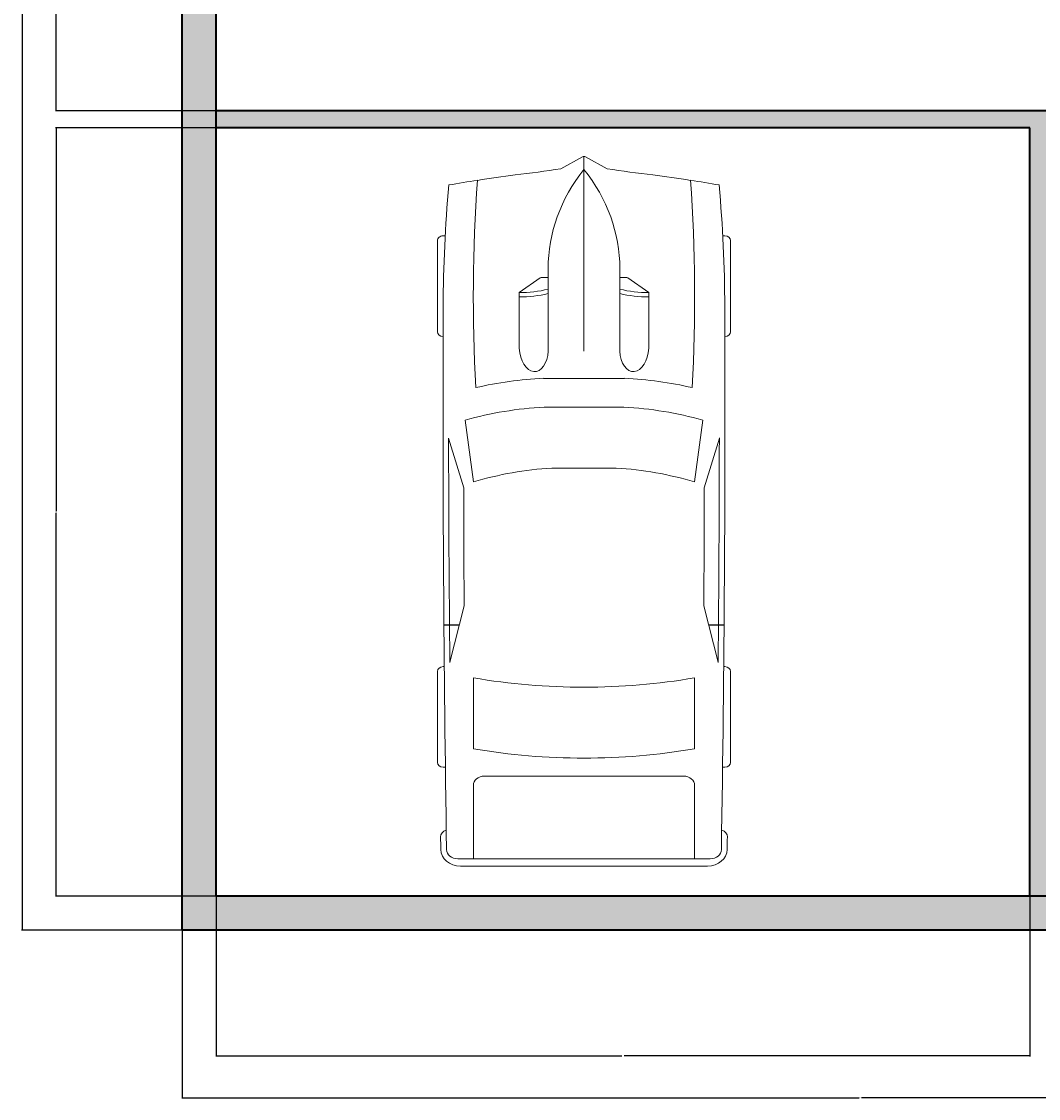
# Model space of a CAD drawing. Units: inches. Extents: x 1563 to 2428, y 777 to 1464.
# Tile 1 of 11: x 1563 to 1832, y 777 to 1063. Entities that reach past the tile are written whole.
import ezdxf

# ---------------------------------------------------------------- set-up
doc = ezdxf.new("R2010")
doc.units = ezdxf.units.IN
for name, color, linetype, lineweight in [('A-ANNO-DIMS', 2, 'Continuous', 18), ('A-FLOR-EDGE', 7, 'Continuous', 25), ('A-SITE-VEHI', 8, 'Continuous', 13), ('A-WALL', 7, 'Continuous', 35), ('A-WALL-PATT', 8, 'Continuous', 13)]:
    doc.layers.add(name, color=color, linetype=linetype, lineweight=lineweight)
doc.styles.get("Standard").update_dxf_attribs({"font": 'arial.ttf'})
doc.dimstyles.get("Standard").update_dxf_attribs({"dimtxt": 0.18, "dimasz": 0.18, "dimexe": 0.18, "dimexo": 0.0625, "dimgap": 0.09, "dimtad": 0, "dimtih": 1, "dimtoh": 1, "dimdec": 4, "dimzin": 0, "dimdsep": 46, "dimtxsty": 'Standard', "dimcen": 0.09, "dimadec": 0, "dimazin": 0, "dimtfac": 1, "dimtdec": 4, "dimtofl": 0, "dimtmove": 0, "dimatfit": 3, "dimfxl": 1, "dimtolj": 1, "dimtzin": 0, "dimarcsym": 0})

# ---------------------------------------------------------------- blocks, each defined once
blk = doc.blocks.new('*U6')
for p, q in [((21.1, 37.41), (21.1, 36.83)), ((46.55, 38.89), (22.35, 38.89)), ((47.8, 37.39), (47.8, 37.41)), ((135.45, 37.07), (135.45, 37.41)), ((136.7, 38.89), (160.9, 38.89)), ((162.15, 37.41), (162.15, 36.77)), ((87.99, 31.87), (74.76, 35.92)), ((134.31, 35.6), (119.29, 31.78)), ((70.03, 31.54), (86.41, 29.35)), ((186.47, -33.5), (186.47, 33.5)), ((188.4, -32.76), (188.4, 32.76)), ((138.42, 29.35), (157.25, 29.35)), ((186.47, 29.35), (167.01, 29.35)), ((164.52, 26.39), (164.52, -26.39)), ((32.27, 11.63), (36.13, 17.17)), ((36.13, 17.17), (50.94, 17.17)), ((29.77, 9.51), (51.68, 9.51)), ((32.12, 9.51), (32.12, 11.15)), ((58.92, -10.77), (58.92, 10.77)), ((66.55, -10.53), (66.55, 10.53)), ((186.47, -10.53), (186.47, 10.53)), ((3.27, 6.13), (0.1, 0.41)), ((82.74, 8.5), (82.74, -8.5)), ((0, 0), (51.68, 0)), ((0.1, -0.41), (3.27, -6.13)), ((29.77, -9.51), (51.68, -9.51)), ((32.12, -9.51), (32.12, -11.15)), ((32.27, -11.63), (36.13, -17.17)), ((36.13, -17.17), (50.94, -17.17)), ((86.41, -29.35), (70.03, -31.54)), ((157.25, -29.35), (138.42, -29.35)), ((167.01, -29.35), (186.47, -29.35)), ((87.99, -31.87), (74.76, -35.92)), ((134.31, -35.6), (119.29, -31.78)), ((21.1, -37.41), (21.1, -36.83)), ((135.45, -37.07), (135.45, -37.41)), ((162.15, -37.41), (162.15, -36.77)), ((46.55, -38.89), (22.35, -38.89)), ((47.8, -37.39), (47.8, -37.41)), ((136.7, -38.89), (160.9, -38.89))]:
    blk.add_line(p, q)
for centre, major_axis, ratio, start_param, end_param in [((41.19, -490.86), (0, 528.23), 0.842304, 0.00281, 0.075598), ((22.35, 37.41), (0, -1.48), 0.842304, 3.141593, 4.712389), ((64.48, -10555.62), (0, 10593.03), 0.842304, -0.013397, 0.002797), ((46.55, 37.41), (0, 1.48), 0.842304, -1.570796, 0), ((136.7, 37.41), (0, -1.48), 0.842304, 3.141593, 4.712389), ((160.9, 37.41), (0, 1.48), 0.842304, -1.570796, 0), ((180.63, 35.84), (0, 2.22), 0.842304, -0.013017, 1.249894), ((64.48, -10556.36), (0, 10595.31), 0.842304, -0.013397, -0.013017), ((183.98, 32.76), (0, -5.25), 0.842304, 1.570796, 3.128196), ((266.03, -27.52), (0, 313.31), 0.842304, 1.367076, 1.39176), ((64.48, -10555.62), (0, -10591.55), 0.842304, 3.133765, 3.140441), ((183.98, 33.5), (0, -2.96), 0.842304, 1.570796, 3.128196), ((135.29, 5.39), (0, 81.77), 0.842304, 1.245306, 1.50788), ((95.79, -3666.35), (0, -3698.24), 0.842304, 3.134049, 3.144098), ((37.47, -593.96), (0, -623.33), 0.842304, 3.096046, 3.200911), ((134.4, 5.39), (0, -89.78), 0.842304, 4.449482, 4.652344), ((149.6, 2.8), (0, -79.58), 0.842304, 4.372215, 4.640744), ((17.08, 0), (0, 147.02), 0.842304, 4.511394, 4.913384), ((35.91, 0), (0, 147.02), 0.842304, 4.511394, 4.913384), ((167.01, 26.39), (0, 2.96), 0.842304, 0, 1.570796), ((259.18, -27.52), (0, -305.3), 0.842304, 4.528606, 4.561838), ((-204.49, 52.4), (0, -250.96), 0.842304, 1.385369, 1.434372), ((13.04, 17.01), (0, 27.42), 0.842304, 4.435146, 4.718221), ((14.2, 17.01), (0, 27.42), 0.842304, 4.435146, 4.718221), ((50.79, 13.34), (6.34, -0.36), 0.603834, -1.395552, 1.581315), ((32.75, 11.15), (0, 0.74), 0.842304, 0.879714, 1.570796), ((29.77, -46.66), (0, 56.17), 0.842304, 0, 0.590319), ((0.62, 0), (0, -0.74), 0.842304, 4.131459, 5.293319), ((29.77, 46.66), (0, 56.17), 0.842304, 2.551274, 3.141593), ((-204.49, -52.4), (0, 250.96), 0.842304, -1.434372, -1.385369), ((149.6, -2.8), (0, -79.58), 0.842304, -1.499151, -1.230623), ((32.75, -11.15), (0, -0.74), 0.842304, 4.712389, 5.403472), ((13.04, -17.01), (0, -27.42), 0.842304, 1.564964, 1.848039), ((14.2, -17.01), (0, -27.42), 0.842304, 1.564964, 1.848039), ((134.4, -5.39), (0, -89.78), 0.842304, -1.510751, -1.307889), ((135.29, -5.39), (0, -81.77), 0.842304, -1.50788, -1.245306), ((259.18, 27.52), (0, 305.3), 0.842304, 1.721348, 1.754579), ((266.03, 27.52), (0, 313.31), 0.842304, 1.749832, 1.774517), ((37.47, 593.96), (0, -623.33), 0.842304, -0.059319, 0.045547), ((167.01, -26.39), (0, -2.96), 0.842304, 4.712389, 6.283185), ((95.79, 3666.35), (0, -3698.24), 0.842304, -0.002505, 0.007544), ((183.98, -33.5), (0, 2.96), 0.842304, 3.15499, 4.712389), ((183.98, -32.76), (0, -5.25), 0.842304, 0.013397, 1.570796), ((41.19, 490.86), (0, -528.23), 0.842304, -0.075598, -0.00281), ((64.48, 10555.62), (0, 10593.03), 0.842304, 3.138796, 3.15499), ((64.48, 10555.62), (0, -10591.55), 0.842304, 0.001152, 0.007828), ((180.63, -35.84), (0, -2.22), 0.842304, -1.249894, 0.013017), ((22.35, -37.41), (0, 1.48), 0.842304, 1.570796, 3.141593), ((46.55, -37.41), (0, -1.48), 0.842304, 0, 1.570796), ((136.7, -37.41), (0, -1.48), 0.842304, -1.570796, 0), ((160.9, -37.41), (0, 1.48), 0.842304, 3.141593, 4.712389), ((64.48, 10556.36), (0, 10595.31), 0.842304, 3.15461, 3.15499)]:
    blk.add_ellipse(centre, major_axis=major_axis, ratio=ratio, start_param=start_param, end_param=end_param)
at = {"extrusion": (0, 0, -1)}
blk.add_ellipse((50.79, -13.34), major_axis=(6.34, 0.36), ratio=0.603834, start_param=-1.395552, end_param=1.581315, dxfattribs=at)
blk = doc.blocks.new('*D48')
at = {"layer": 'A-ANNO-DIMS', "color": 0, "lineweight": -2, "transparency": 16777216}
for p, q in [((1605.11, 821.37), (1605.11, 776.74)), ((1965.11, 821.37), (1965.11, 776.74)), ((1605.29, 776.92), (1784.82, 776.92)), ((1964.93, 776.92), (1785.39, 776.92))]:
    blk.add_line(p, q, dxfattribs=at)
at = {"layer": 'A-ANNO-DIMS', "color": 0, "transparency": 16777216}
for points in [[(1605.29, 776.95), (1605.29, 776.89), (1605.11, 776.92)], [(1964.93, 776.95), (1964.93, 776.89), (1965.11, 776.92)]]:
    blk.add_solid(points, dxfattribs=at)
at = {"layer": 'Defpoints', "color": 0, "transparency": 16777216}
for p in [(1605.11, 821.43), (1965.11, 821.43), (1965.11, 776.92)]:
    blk.add_point(p, dxfattribs=at)
at = {"layer": 'A-ANNO-DIMS', "color": 0, "transparency": 16777216, "insert": (1785.11, 776.92), "char_height": 0.18, "attachment_point": 5}
blk.add_mtext('\\A1;360', dxfattribs=at)
blk = doc.blocks.new('*D49')
at = {"layer": 'A-ANNO-DIMS', "color": 0, "lineweight": -2, "transparency": 16777216}
for p, q in [((1605.04, 1421.43), (1562.53, 1421.43)), ((1562.71, 1421.25), (1562.71, 1121.61)), ((1562.71, 821.61), (1562.71, 1121.25)), ((1605.04, 821.43), (1562.53, 821.43))]:
    blk.add_line(p, q, dxfattribs=at)
at = {"layer": 'A-ANNO-DIMS', "color": 0, "transparency": 16777216}
for points in [[(1562.68, 1421.25), (1562.74, 1421.25), (1562.71, 1421.43)], [(1562.68, 821.61), (1562.74, 821.61), (1562.71, 821.43)]]:
    blk.add_solid(points, dxfattribs=at)
at = {"layer": 'Defpoints', "color": 0, "transparency": 16777216}
for p in [(1562.71, 1421.43), (1605.11, 1421.43), (1605.11, 821.43)]:
    blk.add_point(p, dxfattribs=at)
at = {"layer": 'A-ANNO-DIMS', "color": 0, "transparency": 16777216, "insert": (1562.71, 1121.43), "char_height": 0.18, "attachment_point": 5}
blk.add_mtext('\\A1;600', dxfattribs=at)
blk = doc.blocks.new('*D58')
at = {"layer": 'A-ANNO-DIMS', "color": 0, "lineweight": -2, "transparency": 16777216}
for p, q in [((1614.04, 1199.43), (1571.53, 1199.43)), ((1571.71, 1199.25), (1571.71, 1119.36)), ((1571.71, 1039.11), (1571.71, 1119)), ((1614.04, 1038.93), (1571.53, 1038.93))]:
    blk.add_line(p, q, dxfattribs=at)
at = {"layer": 'A-ANNO-DIMS', "color": 0, "transparency": 16777216}
for points in [[(1571.68, 1199.25), (1571.74, 1199.25), (1571.71, 1199.43)], [(1571.68, 1039.11), (1571.74, 1039.11), (1571.71, 1038.93)]]:
    blk.add_solid(points, dxfattribs=at)
at = {"layer": 'Defpoints', "color": 0, "transparency": 16777216}
for p in [(1571.71, 1199.43), (1614.11, 1199.43), (1614.11, 1038.93)]:
    blk.add_point(p, dxfattribs=at)
at = {"layer": 'A-ANNO-DIMS', "color": 0, "transparency": 16777216, "insert": (1571.71, 1119.18), "char_height": 0.18, "attachment_point": 5}
blk.add_mtext('\\A1;160.5', dxfattribs=at)
blk = doc.blocks.new('*D59')
at = {"layer": 'A-ANNO-DIMS', "color": 0, "lineweight": -2, "transparency": 16777216}
for p, q in [((1614.04, 1034.43), (1571.53, 1034.43)), ((1571.71, 1034.25), (1571.71, 932.61)), ((1571.71, 830.61), (1571.71, 932.25)), ((1614.04, 830.43), (1571.53, 830.43))]:
    blk.add_line(p, q, dxfattribs=at)
at = {"layer": 'A-ANNO-DIMS', "color": 0, "transparency": 16777216}
for points in [[(1571.68, 1034.25), (1571.74, 1034.25), (1571.71, 1034.43)], [(1571.68, 830.61), (1571.74, 830.61), (1571.71, 830.43)]]:
    blk.add_solid(points, dxfattribs=at)
at = {"layer": 'Defpoints', "color": 0, "transparency": 16777216}
for p in [(1571.71, 1034.43), (1614.11, 1034.43), (1614.11, 830.43)]:
    blk.add_point(p, dxfattribs=at)
at = {"layer": 'A-ANNO-DIMS', "color": 0, "transparency": 16777216, "insert": (1571.71, 932.43), "char_height": 0.18, "attachment_point": 5}
blk.add_mtext('\\A1;204', dxfattribs=at)
blk = doc.blocks.new('*D60')
at = {"layer": 'A-ANNO-DIMS', "color": 0, "lineweight": -2, "transparency": 16777216}
for p, q in [((1614.11, 830.37), (1614.11, 787.85)), ((1830.11, 830.37), (1830.11, 787.85)), ((1614.29, 788.03), (1721.82, 788.03)), ((1829.93, 788.03), (1722.4, 788.03))]:
    blk.add_line(p, q, dxfattribs=at)
at = {"layer": 'A-ANNO-DIMS', "color": 0, "transparency": 16777216}
for points in [[(1614.29, 788.06), (1614.29, 788), (1614.11, 788.03)], [(1829.93, 788.06), (1829.93, 788), (1830.11, 788.03)]]:
    blk.add_solid(points, dxfattribs=at)
at = {"layer": 'Defpoints', "color": 0, "transparency": 16777216}
for p in [(1614.11, 830.43), (1830.11, 830.43), (1614.11, 788.03)]:
    blk.add_point(p, dxfattribs=at)
at = {"layer": 'A-ANNO-DIMS', "color": 0, "transparency": 16777216, "insert": (1722.11, 788.03), "char_height": 0.18, "attachment_point": 5}
blk.add_mtext('\\A1;216', dxfattribs=at)

msp = doc.modelspace()

# ---------------------------------------------------------------- hatches: boundary and pattern name
at = {"layer": 'A-WALL-PATT'}
h = msp.add_hatch(color=256, dxfattribs=at)
h.dxf.hatch_style = 1
h.paths.add_polyline_path([(1965.105, 1421.428), (1605.105, 1421.428), (1605.105, 821.428), (1965.105, 821.428)])
h.paths.add_polyline_path([(1614.105, 1199.428), (1704.105, 1199.428), (1738.605, 1199.428), (1738.605, 1251.928), (1734.105, 1251.928), (1734.105, 1203.928), (1704.105, 1203.928), (1614.105, 1203.928), (1614.105, 1335.928), (1665.105, 1335.928), (1665.105, 1340.428), (1614.105, 1340.428), (1614.105, 1412.428), (1704.105, 1412.428), (1704.105, 1340.428), (1701.105, 1340.428), (1701.105, 1335.928), (1704.105, 1335.928), (1768.605, 1335.928), (1768.605, 1340.428), (1708.605, 1340.428), (1708.605, 1412.428), (1807.605, 1412.428), (1807.605, 1340.428), (1804.605, 1340.428), (1804.605, 1335.928), (1807.605, 1335.928), (1807.605, 1275.928), (1815.105, 1275.928), (1815.105, 1280.428), (1812.105, 1280.428), (1812.105, 1412.428), (1956.105, 1412.428), (1956.105, 1280.428), (1854.105, 1280.428), (1854.105, 1275.928), (1956.105, 1275.928), (1956.105, 830.428), (1614.105, 830.428)], flags=16)
h.paths.add_polyline_path([(1917.224, 1038.928), (1917.224, 1043.846, -0.4014527), (1951.591, 1079.751), (1951.591, 1079.786), (1953.163, 1079.786), (1953.163, 1043.846), (1953.163, 1038.455), (1953.105, 1034.428), (1953.105, 1038.928), (1953.163, 1043.846), (1951.591, 1043.846), (1951.591, 1079.751, 0.4014527), (1917.224, 1043.846), (1917.224, 1038.455), (1917.224, 1034.428), (1834.605, 1034.428), (1834.605, 906.928), (1858.605, 906.928), (1858.605, 954.928), (1932.105, 954.928), (1932.105, 902.428), (1834.605, 902.428), (1834.605, 1034.428), (1914.224, 1034.428), (1914.224, 1038.928)], flags=0)
edge = h.paths.add_edge_path(flags=0)
edge.add_ellipse((1674.345, 1004.483), major_axis=(1.48, 0), ratio=0.8423039, start_angle=90, end_angle=180, ccw=False)
edge.add_line((1674.345, 1005.73), (1674.921, 1005.73))
edge.add_ellipse((2202.617, 985.642), major_axis=(528.234, 0), ratio=0.8423039, start_angle=176.34957, end_angle=177.82005, ccw=False)
edge.add_ellipse((1739.278, 760.804), major_axis=(-313.308, 0), ratio=0.8423039, start_angle=-77.87403, end_angle=-76.21947, ccw=False)
edge.add_ellipse((1739.278, 767.659), major_axis=(305.303, 0), ratio=0.8423039, start_angle=100.20954, end_angle=102.44463, ccw=False)
edge.add_ellipse((1659.357, 1231.328), major_axis=(250.96, 0), ratio=0.8423039, start_angle=-80.74343, end_angle=-77.44507)
edge.add_line((1705.625, 1023.567), (1711.685, 1026.918))
edge.add_ellipse((1711.754, 1026.21), major_axis=(0.74, 0), ratio=0.8423039, start_angle=52.06687, end_angle=90, ccw=False)
edge.add_line((1712.16, 1026.731), (1717.882, 1023.567))
edge.add_ellipse((1764.151, 1231.328), major_axis=(250.96, 0), ratio=0.8423039, start_angle=257.44507, end_angle=260.74343)
edge.add_ellipse((1684.229, 767.659), major_axis=(305.303, 0), ratio=0.8423039, start_angle=77.55537, end_angle=79.79046, ccw=False)
edge.add_ellipse((1684.229, 760.804), major_axis=(-313.308, 0), ratio=0.8423039, start_angle=256.21947, end_angle=257.87403, ccw=False)
edge.add_ellipse((1220.891, 985.642), major_axis=(-528.234, 0), ratio=0.8423039, start_angle=182.17995, end_angle=183.65043, ccw=False)
edge.add_line((1748.586, 1005.73), (1749.162, 1005.73))
edge.add_ellipse((1749.162, 1004.483), major_axis=(-1.48, 0), ratio=0.8423039, start_angle=180, end_angle=270, ccw=False)
edge.add_line((1750.642, 1004.483), (1750.642, 980.28))
edge.add_ellipse((1749.162, 980.28), major_axis=(1.48, 0), ratio=0.8423039, start_angle=270, end_angle=360, ccw=False)
edge.add_ellipse((-8843.864, 962.352), major_axis=(10593.026, 0), ratio=0.84230387, start_angle=-0.3241203, end_angle=0.0902291, ccw=False)
edge.add_ellipse((-8843.864, 962.352), major_axis=(10593.026, 0), ratio=0.84230387, start_angle=-0.3838668, end_angle=-0.3241203, ccw=False)
edge.add_ellipse((1749.162, 890.136), major_axis=(1.48, 0), ratio=0.8423039, start_angle=0, end_angle=90, ccw=False)
edge.add_line((1750.642, 890.136), (1750.642, 865.933))
edge.add_ellipse((1749.162, 865.933), major_axis=(1.48, 0), ratio=0.8423039, start_angle=270, end_angle=360, ccw=False)
edge.add_line((1749.162, 864.686), (1748.528, 864.686))
edge.add_ellipse((-8843.864, 962.352), major_axis=(10593.026, 0), ratio=0.84230387, start_angle=-0.6186432, end_angle=-0.5282715, ccw=False)
edge.add_ellipse((1747.592, 846.206), major_axis=(-2.22, 0), ratio=0.8423039, start_angle=179.37176, end_angle=248.46476, ccw=False)
edge.add_ellipse((-8844.604, 962.352), major_axis=(-10595.313, 0), ratio=0.842303864, start_angle=179.3534459, end_angle=179.3717628, ccw=False)
edge.add_ellipse((1744.512, 842.854), major_axis=(-5.246, 0), ratio=0.8423039, start_angle=90, end_angle=179.35345, ccw=False)
edge.add_line((1744.512, 838.435), (1678.995, 838.435))
edge.add_ellipse((1678.995, 842.854), major_axis=(5.246, 0), ratio=0.8423039, start_angle=180.64655, end_angle=270, ccw=False)
edge.add_ellipse((12268.111, 962.352), major_axis=(-10595.313, 0), ratio=0.84230387, start_angle=0.6282372, end_angle=0.6465541, ccw=False)
edge.add_ellipse((1675.916, 846.206), major_axis=(-2.22, 0), ratio=0.8423039, start_angle=-68.46476, end_angle=0.62824, ccw=False)
edge.add_ellipse((12267.371, 962.352), major_axis=(-10593.026, 0), ratio=0.84230387, start_angle=0.5282715, end_angle=0.6465541, ccw=False)
edge.add_line((1674.98, 864.686), (1674.345, 864.686))
edge.add_ellipse((1674.345, 865.933), major_axis=(-1.48, 0), ratio=0.8423039, start_angle=0, end_angle=90, ccw=False)
edge.add_line((1672.865, 865.933), (1672.865, 890.136))
edge.add_ellipse((1674.345, 890.136), major_axis=(1.48, 0), ratio=0.8423039, start_angle=90, end_angle=180, ccw=False)
edge.add_ellipse((12267.371, 962.352), major_axis=(-10593.026, 0), ratio=0.84230387, start_angle=0.3241203, end_angle=0.3838668, ccw=False)
edge.add_ellipse((12267.371, 962.352), major_axis=(-10593.026, 0), ratio=0.84230387, start_angle=-0.0902291, end_angle=0.3241203, ccw=False)
edge.add_ellipse((1674.345, 980.28), major_axis=(-1.48, 0), ratio=0.8423039, start_angle=0, end_angle=90, ccw=False)
edge.add_line((1672.865, 980.28), (1672.865, 1004.483))
h.paths.add_polyline_path([(1622.542, 1135.584), (1648.534, 1136.233), (1648.683, 1130.234), (1647.126, 1130.196), (1648.323, 1082.21), (1649.88, 1082.249), (1650.03, 1076.251), (1624.038, 1075.603, -0.266667)], flags=0)
edge = h.paths.add_edge_path(flags=0)
edge.add_line((1694.584, 990.705), (1700.334, 994.711))
edge.add_line((1700.334, 994.711), (1702.248, 994.711))
edge.add_line((1702.248, 994.711), (1702.248, 997.061))
edge.add_ellipse((1758.417, 997.061), major_axis=(56.169, 0), ratio=0.8423039, start_angle=150.56143, end_angle=180, ccw=False)
edge.add_ellipse((1665.091, 997.061), major_axis=(-56.169, 0), ratio=0.8423039, start_angle=180, end_angle=209.43857, ccw=False)
edge.add_line((1721.26, 997.061), (1721.26, 994.711))
edge.add_line((1721.26, 994.711), (1723.174, 994.711))
edge.add_line((1723.174, 994.711), (1728.923, 990.705))
edge.add_line((1728.923, 990.705), (1728.923, 975.895))
edge.add_ellipse((1725.091, 976.043), major_axis=(0.357, 6.34), ratio=0.6038336, start_angle=106.34259, end_angle=270.99799, ccw=False)
edge.add_line((1721.26, 975.15), (1721.26, 997.061))
edge.add_ellipse((1665.091, 997.061), major_axis=(-56.169, 0), ratio=0.8423039, start_angle=180, end_angle=209.43857)
edge.add_ellipse((1758.417, 997.061), major_axis=(56.169, 0), ratio=0.8423039, start_angle=150.56143, end_angle=180)
edge.add_line((1702.248, 997.061), (1702.248, 975.15))
edge.add_ellipse((1698.416, 976.043), major_axis=(-0.357, 6.34), ratio=0.6038336, start_angle=89.00201, end_angle=253.65741, ccw=False)
edge.add_line((1694.584, 975.895), (1694.584, 990.705))
edge = h.paths.add_edge_path(flags=0)
edge.add_line((1675.832, 952.075), (1679.883, 938.848))
edge.add_ellipse((5378.107, 931.045), major_axis=(-3698.236, 0), ratio=0.84230387, start_angle=-0.120897, end_angle=0.364076)
edge.add_line((1679.976, 907.545), (1676.149, 892.52))
edge.add_ellipse((12267.371, 962.352), major_axis=(10591.546, 0), ratio=0.84230387, start_angle=180.3241656, end_angle=180.3777642, ccw=False)
edge.add_ellipse((12267.371, 962.352), major_axis=(10591.546, 0), ratio=0.84230387, start_angle=180.0555943, end_angle=180.3241656, ccw=False)
edge = h.paths.add_edge_path(flags=0)
edge.add_ellipse((1706.366, 891.542), major_axis=(81.773, 0), ratio=0.8423039, start_angle=94.27742, end_angle=111.83495, ccw=False)
edge.add_line((1701.225, 960.283), (1722.283, 960.283))
edge.add_ellipse((1717.141, 891.542), major_axis=(-81.773, 0), ratio=0.8423039, start_angle=248.16505, end_angle=265.72258, ccw=False)
edge.add_line((1743.29, 956.803), (1741.105, 940.427))
edge.add_ellipse((1714.553, 877.238), major_axis=(79.58, 0), ratio=0.8423039, start_angle=67.20809, end_angle=85.12993)
edge.add_line((1720.25, 944.097), (1703.258, 944.097))
edge.add_ellipse((1708.954, 877.238), major_axis=(79.58, 0), ratio=0.8423039, start_angle=94.87007, end_angle=112.79191)
edge.add_line((1682.403, 940.427), (1680.218, 956.803))
h.paths.add_polyline_path([(1664.992, 1093.991), (1664.992, 1123.991), (1724.992, 1123.991), (1724.992, 1093.991)], flags=0)
h.paths.add_polyline_path([(1716.588, 1099.729), (1715.404, 1099.805), (1715.021, 1099.823), (1716.177, 1099.758)], flags=0)
h.paths.add_polyline_path([(1711.325, 1103.757), (1712.167, 1103.706), (1713.009, 1103.642), (1713.84, 1103.566), (1715.041, 1103.439), (1716.532, 1103.244), (1717.793, 1103.048), (1718.876, 1102.854), (1719.676, 1102.699), (1720.157, 1102.605), (1720.632, 1102.513), (1721.109, 1102.424), (1721.595, 1102.339), (1722.088, 1102.264), (1722.585, 1102.205), (1723.082, 1102.17), (1723.575, 1102.164), (1724.321, 1102.211), (1724.533, 1102.268), (1723.842, 1102.16), (1722.864, 1102.172), (1721.894, 1102.287), (1720.935, 1102.454), (1720.157, 1102.605), (1719.676, 1102.699), (1719.18, 1102.795), (1718.66, 1102.892), (1718.109, 1102.991), (1717.517, 1103.091), (1716.876, 1103.191), (1716.179, 1103.29), (1715.435, 1103.387), (1714.652, 1103.48), (1713.84, 1103.566), (1713.009, 1103.642), (1712.167, 1103.706), (1711.325, 1103.757), (1710.492, 1103.791), (1709.676, 1103.806), (1708.873, 1103.805), (1707.707, 1103.78), (1707.292, 1103.757), (1708.499, 1103.805), (1710.086, 1103.807)], flags=0)
h.paths.add_polyline_path([(1713.959, 1106.591), (1714.651, 1106.624), (1715.279, 1106.674), (1715.852, 1106.736), (1716.373, 1106.807), (1716.851, 1106.885), (1717.289, 1106.966), (1717.696, 1107.046), (1718.341, 1107.178), (1719.173, 1107.331), (1720.169, 1107.421), (1721.131, 1107.383), (1722.032, 1107.286), (1722.934, 1107.152), (1723.887, 1106.983), (1724.746, 1106.795), (1724.72, 1106.798), (1724.663, 1106.807), (1724.241, 1106.906), (1724.159, 1106.924), (1723.885, 1106.979), (1723.546, 1107.044), (1723.157, 1107.113), (1722.732, 1107.182), (1722.284, 1107.249), (1721.827, 1107.308), (1721.375, 1107.357), (1720.942, 1107.391), (1720.539, 1107.406), (1720.162, 1107.405), (1719.804, 1107.388), (1719.459, 1107.357), (1719.12, 1107.314), (1718.781, 1107.259), (1718.435, 1107.195), (1718.076, 1107.124), (1717.402, 1106.986), (1716.59, 1106.837), (1715.56, 1106.696), (1714.317, 1106.598)], flags=0)
h.paths.add_polyline_path([(1708.692, 1110.124), (1709.455, 1110.13), (1710.147, 1110.149), (1710.772, 1110.18), (1711.334, 1110.224), (1711.836, 1110.28), (1712.283, 1110.349), (1712.678, 1110.43), (1713.026, 1110.524), (1713.33, 1110.63), (1713.596, 1110.746), (1713.832, 1110.87), (1714.042, 1110.999), (1714.234, 1111.131), (1714.413, 1111.264), (1714.586, 1111.396), (1715.065, 1111.75), (1715.879, 1112.11), (1716.842, 1112.224), (1717.903, 1112.165), (1719.048, 1111.965), (1719.867, 1111.736), (1720.686, 1111.487), (1721.596, 1111.22), (1721.917, 1111.136), (1721.028, 1111.383), (1720.222, 1111.628), (1719.815, 1111.75), (1719.434, 1111.857), (1719.054, 1111.951), (1718.672, 1112.031), (1718.292, 1112.097), (1717.918, 1112.149), (1717.554, 1112.185), (1717.204, 1112.204), (1716.871, 1112.206), (1716.559, 1112.191), (1716.271, 1112.156), (1716.006, 1112.105), (1715.761, 1112.038), (1715.534, 1111.957), (1715.323, 1111.864), (1715.125, 1111.759), (1714.937, 1111.645), (1714.759, 1111.524), (1714.586, 1111.396), (1714.413, 1111.264), (1714.003, 1110.96), (1713.331, 1110.606), (1712.501, 1110.382), (1711.61, 1110.245), (1710.489, 1110.158), (1709.111, 1110.121)], flags=0)
h.paths.add_polyline_path([(1707.127, 1113.075), (1707.639, 1113.025), (1708.092, 1112.991), (1708.49, 1112.975), (1708.836, 1112.977), (1709.135, 1112.996), (1709.392, 1113.032), (1709.612, 1113.084), (1709.798, 1113.15), (1709.957, 1113.23), (1710.092, 1113.324), (1710.208, 1113.431), (1710.304, 1113.554), (1710.379, 1113.698), (1710.434, 1113.866), (1710.467, 1114.062), (1710.477, 1114.289), (1710.463, 1114.553), (1710.426, 1114.857), (1710.364, 1115.202), (1710.282, 1115.58), (1710.184, 1115.98), (1710.076, 1116.391), (1709.961, 1116.801), (1709.844, 1117.201), (1709.731, 1117.579), (1709.626, 1117.924), (1709.532, 1118.228), (1709.454, 1118.493), (1709.392, 1118.723), (1709.351, 1118.924), (1709.293, 1119.435), (1709.831, 1119.942), (1710.705, 1120.121), (1711.507, 1119.898), (1712.224, 1119.567), (1713.189, 1119.016), (1713.529, 1118.804), (1712.958, 1119.148), (1712.468, 1119.428), (1712.046, 1119.649), (1711.683, 1119.817), (1711.366, 1119.937), (1711.084, 1120.016), (1710.826, 1120.057), (1710.582, 1120.067), (1710.354, 1120.049), (1710.142, 1120.006), (1709.951, 1119.941), (1709.781, 1119.857), (1709.635, 1119.757), (1709.516, 1119.645), (1709.426, 1119.524), (1709.366, 1119.395), (1709.335, 1119.255), (1709.331, 1119.1), (1709.351, 1118.924), (1709.392, 1118.723), (1709.454, 1118.493), (1709.52, 1118.268), (1709.799, 1117.356), (1710.028, 1116.57), (1710.245, 1115.749), (1710.45, 1114.804), (1710.477, 1114.289), (1710.448, 1113.654), (1709.908, 1113.153), (1709.165, 1112.979), (1708.318, 1112.974), (1707.448, 1113.039)], flags=0)
h.paths.add_polyline_path([(1700.892, 1119.857), (1701.604, 1119.819), (1702.196, 1119.805), (1702.683, 1119.813), (1703.076, 1119.841), (1703.387, 1119.887), (1703.63, 1119.951), (1703.816, 1120.03), (1703.959, 1120.124), (1704.069, 1120.23), (1704.15, 1120.346), (1704.204, 1120.47), (1704.234, 1120.599), (1704.242, 1120.731), (1704.231, 1120.864), (1704.202, 1120.996), (1704.159, 1121.124), (1704.103, 1121.246), (1704.039, 1121.362), (1703.97, 1121.474), (1703.901, 1121.582), (1703.834, 1121.687), (1703.775, 1121.79), (1703.564, 1122.226), (1704.048, 1122.698), (1704.756, 1122.769), (1705.49, 1122.723), (1706.24, 1122.641), (1706.547, 1122.601), (1706.092, 1122.657), (1705.695, 1122.701), (1705.348, 1122.732), (1705.049, 1122.751), (1704.792, 1122.757), (1704.573, 1122.751), (1704.386, 1122.732), (1704.227, 1122.701), (1704.092, 1122.657), (1703.977, 1122.601), (1703.88, 1122.534), (1703.802, 1122.458), (1703.742, 1122.374), (1703.702, 1122.284), (1703.68, 1122.188), (1703.677, 1122.09), (1703.692, 1121.991), (1703.726, 1121.89), (1703.769, 1121.802), (1704.039, 1121.362), (1704.301, 1120.887), (1704.133, 1120.165), (1703.43, 1119.866), (1702.481, 1119.798), (1701.306, 1119.827)], flags=0)
edge = h.paths.add_edge_path(flags=0)
edge.add_ellipse((1711.754, 1009.752), major_axis=(-147.018, 0), ratio=0.8423039, start_angle=76.40187, end_angle=103.59813)
edge.add_line((1741.105, 888.411), (1741.105, 869.587))
edge.add_ellipse((1711.754, 990.928), major_axis=(-147.018, 0), ratio=0.8423039, start_angle=76.40187, end_angle=103.59813, ccw=False)
edge.add_line((1682.403, 869.587), (1682.403, 888.411))
edge = h.paths.add_edge_path(flags=0)
edge.add_ellipse((-8843.864, 962.352), major_axis=(-10591.546, 0), ratio=0.84230387, start_angle=179.6758344, end_angle=179.9444057, ccw=False)
edge.add_ellipse((-8843.864, 962.352), major_axis=(-10591.546, 0), ratio=0.84230387, start_angle=179.6222358, end_angle=179.6758344, ccw=False)
edge.add_line((1747.358, 892.52), (1743.531, 907.545))
edge.add_ellipse((-1954.6, 931.045), major_axis=(3698.236, 0), ratio=0.84230387, start_angle=-0.364076, end_angle=0.120897)
edge.add_line((1743.625, 938.848), (1747.676, 952.075))
h.paths.add_polyline_path([(1637.931, 1162.087), (1637.931, 1188.087, -0.1904762), (1721.931, 1188.087), (1721.931, 1162.087), (1715.931, 1162.087), (1715.931, 1163.644), (1643.931, 1163.644), (1643.931, 1162.087)], flags=0)
h.paths.add_polyline_path([(1667.931, 1189.491, -0.0496282), (1691.931, 1189.491), (1691.931, 1182.705), (1667.931, 1182.705)], flags=0)
edge = h.paths.add_edge_path(flags=0)
edge.add_ellipse((1685.362, 859.825), major_axis=(-2.96, 0), ratio=0.8423039, start_angle=-90, end_angle=0, ccw=False)
edge.add_line((1685.362, 862.318), (1738.145, 862.318))
edge.add_ellipse((1738.145, 859.825), major_axis=(2.96, 0), ratio=0.8423039, start_angle=0, end_angle=90, ccw=False)
edge.add_line((1741.105, 859.825), (1741.105, 840.361))
edge.add_line((1741.105, 840.361), (1682.403, 840.361))
edge.add_line((1682.403, 840.361), (1682.403, 859.825))
h.paths.add_polyline_path([(1777.486, 1164.853), (1777.486, 1180.853), (1778.486, 1181.01), (1778.486, 1164.697)], flags=0)
h.paths.add_polyline_path([(1786.986, 1154.853), (1786.986, 1163.369), (1778.986, 1164.619), (1778.986, 1181.088), (1786.986, 1182.338), (1786.986, 1190.853), (1799.502, 1190.853), (1800.752, 1198.853), (1817.221, 1198.853), (1818.471, 1190.853), (1827.502, 1190.853), (1828.752, 1198.853), (1845.221, 1198.853), (1846.471, 1190.853), (1858.986, 1190.853), (1858.986, 1182.338), (1866.986, 1181.088), (1866.986, 1164.619), (1858.986, 1163.369), (1858.986, 1154.853), (1846.471, 1154.853), (1845.221, 1146.853), (1828.752, 1146.853), (1827.502, 1154.853), (1818.471, 1154.853), (1817.221, 1146.853), (1800.752, 1146.853), (1799.502, 1154.853)], flags=0)
h.paths.add_polyline_path([(1800.986, 1145.353), (1800.83, 1146.353), (1817.143, 1146.353), (1816.986, 1145.353)], flags=0)
h.paths.add_polyline_path([(1851.408, 1167.858), (1852.086, 1167.738), (1852.744, 1167.621), (1853.388, 1167.506), (1854.028, 1167.395), (1854.67, 1167.289), (1855.313, 1167.195), (1855.952, 1167.122), (1856.585, 1167.077), (1857.209, 1167.07), (1858.147, 1167.128), (1858.413, 1167.2), (1857.547, 1167.066), (1856.312, 1167.08), (1855.07, 1167.223), (1854.028, 1167.395), (1853.388, 1167.506), (1852.744, 1167.621), (1852.086, 1167.738), (1851.408, 1167.858), (1850.288, 1168.052), (1849.956, 1168.104), (1850.701, 1167.98)], flags=0)
h.paths.add_polyline_path([(1845.435, 1172.646), (1846.222, 1172.707), (1846.941, 1172.785), (1847.601, 1172.874), (1848.21, 1172.971), (1848.777, 1173.072), (1849.311, 1173.173), (1850.14, 1173.331), (1851.063, 1173.483), (1852.014, 1173.591), (1853.012, 1173.633), (1854.075, 1173.594), (1855.251, 1173.473), (1856.4, 1173.306), (1857.391, 1173.132), (1857.945, 1173.02), (1858.196, 1172.965), (1858.595, 1172.871), (1858.575, 1172.874), (1858.49, 1172.894), (1858.371, 1172.924), (1858.196, 1172.965), (1857.945, 1173.02), (1857.602, 1173.089), (1857.177, 1173.17), (1856.687, 1173.256), (1856.148, 1173.343), (1855.575, 1173.426), (1854.986, 1173.5), (1854.395, 1173.561), (1853.82, 1173.603), (1853.272, 1173.623), (1852.749, 1173.622), (1852.247, 1173.6), (1851.757, 1173.562), (1851.276, 1173.507), (1850.796, 1173.439), (1850.313, 1173.359), (1849.82, 1173.27), (1849.311, 1173.173), (1848.421, 1173.005), (1847.25, 1172.818), (1845.826, 1172.665)], flags=0)
h.paths.add_polyline_path([(1840.587, 1177.09), (1841.289, 1177.145), (1841.916, 1177.215), (1842.475, 1177.301), (1842.969, 1177.403), (1843.403, 1177.52), (1843.783, 1177.652), (1844.117, 1177.797), (1844.411, 1177.952), (1844.674, 1178.114), (1844.914, 1178.279), (1845.138, 1178.446), (1845.644, 1178.831), (1846.285, 1179.221), (1847.125, 1179.521), (1847.998, 1179.624), (1848.834, 1179.619), (1849.768, 1179.529), (1850.775, 1179.363), (1851.78, 1179.14), (1852.111, 1179.053), (1851.57, 1179.187), (1851.043, 1179.304), (1850.527, 1179.404), (1850.024, 1179.487), (1849.539, 1179.551), (1849.072, 1179.596), (1848.628, 1179.62), (1848.21, 1179.623), (1847.82, 1179.603), (1847.46, 1179.561), (1847.128, 1179.497), (1846.822, 1179.413), (1846.539, 1179.312), (1846.274, 1179.195), (1846.027, 1179.064), (1845.793, 1178.922), (1845.57, 1178.77), (1845.354, 1178.61), (1844.817, 1178.201), (1844.106, 1177.764), (1843.208, 1177.452), (1842.225, 1177.25), (1840.973, 1177.11)], flags=0)
h.paths.add_polyline_path([(1836.67, 1180.646), (1837.236, 1180.603), (1837.734, 1180.584), (1838.166, 1180.586), (1838.54, 1180.611), (1838.861, 1180.655), (1839.136, 1180.72), (1839.369, 1180.803), (1839.568, 1180.903), (1839.736, 1181.02), (1839.881, 1181.152), (1840.001, 1181.299), (1840.095, 1181.456), (1840.164, 1181.624), (1840.204, 1181.8), (1840.217, 1181.981), (1840.2, 1182.166), (1840.153, 1182.353), (1840.076, 1182.541), (1839.973, 1182.728), (1839.851, 1182.916), (1839.716, 1183.103), (1839.572, 1183.291), (1839.427, 1183.478), (1839.033, 1184), (1838.862, 1184.411), (1838.695, 1184.99), (1839.2, 1185.669), (1840.06, 1185.961), (1840.793, 1185.931), (1841.454, 1185.77), (1842.179, 1185.536), (1842.706, 1185.363), (1843.713, 1185.044), (1844.033, 1184.956), (1843.102, 1185.234), (1842.179, 1185.536), (1841.725, 1185.682), (1841.328, 1185.801), (1840.976, 1185.886), (1840.653, 1185.937), (1840.349, 1185.949), (1840.063, 1185.926), (1839.799, 1185.872), (1839.559, 1185.791), (1839.347, 1185.686), (1839.165, 1185.562), (1839.016, 1185.422), (1838.903, 1185.27), (1838.828, 1185.11), (1838.79, 1184.943), (1838.784, 1184.77), (1838.809, 1184.593), (1838.862, 1184.411), (1838.938, 1184.227), (1839.036, 1184.041), (1839.153, 1183.853), (1839.285, 1183.666), (1839.427, 1183.478), (1839.572, 1183.291), (1839.716, 1183.103), (1839.851, 1182.916), (1840.178, 1182.415), (1840.251, 1181.604), (1839.686, 1180.915), (1838.893, 1180.633), (1837.976, 1180.574), (1837.01, 1180.612)], flags=0)
h.paths.add_polyline_path([(1829.867, 1185.622), (1830.475, 1185.631), (1830.966, 1185.666), (1831.355, 1185.724), (1831.658, 1185.804), (1831.891, 1185.903), (1832.07, 1186.02), (1832.207, 1186.152), (1832.308, 1186.297), (1832.376, 1186.452), (1832.414, 1186.614), (1832.424, 1186.779), (1832.41, 1186.946), (1832.374, 1187.11), (1832.32, 1187.27), (1832.25, 1187.422), (1832.17, 1187.568), (1832.084, 1187.708), (1831.997, 1187.843), (1831.914, 1187.974), (1831.839, 1188.102), (1831.614, 1188.57), (1832.036, 1189.169), (1832.801, 1189.319), (1833.589, 1189.3), (1834.44, 1189.223), (1834.736, 1189.187), (1834.239, 1189.241), (1833.807, 1189.28), (1833.433, 1189.304), (1833.111, 1189.312), (1832.837, 1189.304), (1832.604, 1189.28), (1832.405, 1189.241), (1832.236, 1189.187), (1832.092, 1189.117), (1831.971, 1189.033), (1831.873, 1188.938), (1831.799, 1188.832), (1831.748, 1188.719), (1831.721, 1188.601), (1831.717, 1188.478), (1831.736, 1188.353), (1831.779, 1188.228), (1831.839, 1188.102), (1831.914, 1187.974), (1831.997, 1187.843), (1832.084, 1187.708), (1832.387, 1187.216), (1832.456, 1186.393), (1831.916, 1185.871), (1831.195, 1185.682), (1830.221, 1185.613)], flags=0)
h.paths.add_polyline_path([(1828.986, 1145.353), (1828.83, 1146.353), (1845.143, 1146.353), (1844.986, 1145.353)], flags=0)
h.paths.add_polyline_path([(1800.986, 1200.353), (1816.986, 1200.353), (1817.143, 1199.353), (1800.83, 1199.353)], flags=0)
h.paths.add_polyline_path([(1828.986, 1200.353), (1844.986, 1200.353), (1845.143, 1199.353), (1828.83, 1199.353)], flags=0)
h.paths.add_polyline_path([(1867.486, 1181.01), (1868.486, 1180.853), (1868.486, 1164.853), (1867.486, 1164.697)], flags=0)
h.paths.add_polyline_path([(1901.055, 1112.089), (1901.055, 1241.889), (1954.299, 1241.889), (1954.299, 1112.089)], flags=0)
h.paths.add_polyline_path([(1908.544, 1229.408), (1931.009, 1229.408), (1937.23, 1216.927), (1931.009, 1216.927), (1931.009, 1129.562), (1908.544, 1129.562)], flags=0)
h.paths.add_polyline_path([(1699.472, 1381.538), (1701.045, 1381.538), (1701.045, 1345.599), (1699.472, 1345.599)], flags=0)
h.paths.add_polyline_path([(1851.045, 1285.819), (1851.045, 1280.428), (1851.105, 1275.928), (1851.105, 1280.428)], flags=0)
h.paths.add_polyline_path([(1815.105, 1285.819), (1815.105, 1321.758), (1816.678, 1321.758), (1816.678, 1285.819)], flags=0)
h.paths.add_polyline_path([(1745.154, 1343.707, -0.1044693), (1742.568, 1347.148, -0.1176343), (1741.799, 1350.905, -0.1176343), (1742.808, 1354.603, -0.1044693), (1745.61, 1357.871, -0.0900158), (1749.544, 1359.891, -0.0819199), (1754.355, 1360.526, -0.0819199), (1759.115, 1359.583, -0.0900158), (1762.911, 1357.314, -0.1044693), (1765.497, 1353.872, -0.1176343), (1766.266, 1350.116, -0.1176343), (1765.257, 1346.417, -0.1044693), (1762.455, 1343.149, -0.0900158), (1758.521, 1341.13, -0.0819199), (1753.71, 1340.495, -0.0819199), (1748.95, 1341.438, -0.0900158)], flags=0)
h.paths.add_polyline_path([(1745.961, 1344.152, -0.1046782), (1743.517, 1347.257, -0.1186217), (1742.746, 1350.669, -0.1186217), (1743.612, 1354.059, -0.1046782), (1746.143, 1357.094, -0.0895621), (1749.732, 1359.002, -0.0811847), (1754.161, 1359.662, -0.0811847), (1758.57, 1358.877, -0.0895621), (1762.104, 1356.869, -0.1046782), (1764.548, 1353.764, -0.1186217), (1765.319, 1350.351, -0.1186217), (1764.453, 1346.962, -0.1046782), (1761.922, 1343.927, -0.0895621), (1758.333, 1342.019, -0.0811847), (1753.904, 1341.359, -0.0811847), (1749.495, 1342.143, -0.0895621)], flags=0)
h.paths.add_polyline_path([(1748.738, 1346.3, -0.1046075), (1747.125, 1348.343, -0.1182826), (1746.612, 1350.593, -0.1182826), (1747.176, 1352.832, -0.1046075), (1748.833, 1354.838, -0.089718), (1751.19, 1356.103, -0.0814361), (1754.1, 1356.547, -0.0814361), (1756.999, 1356.038, -0.089718), (1759.327, 1354.72, -0.1046075), (1760.94, 1352.678, -0.1182826), (1761.453, 1350.427, -0.1182826), (1760.889, 1348.189, -0.1046075), (1759.232, 1346.183, -0.089718), (1756.875, 1344.917, -0.0814361), (1753.965, 1344.474, -0.0814361), (1751.066, 1344.982, -0.089718)], flags=0)
h.paths.add_polyline_path([(1802.972, 1381.538), (1804.545, 1381.538), (1804.545, 1345.599), (1802.972, 1345.599)], flags=0)
h.paths.add_polyline_path([(1752.533, 1350.51, -1), (1755.533, 1350.51, -1)], flags=0)
h.paths.add_polyline_path([(1753.033, 1350.51, -1), (1755.033, 1350.51, -1)], flags=0)
h.paths.add_polyline_path([(1869.759, 1336.236), (1869.759, 1396.236), (1949.759, 1396.236), (1949.759, 1336.236)], flags=0)
h.paths.add_polyline_path([(1920.159, 1336.236), (1920.159, 1351.436), (1935.359, 1351.436), (1935.359, 1388.236), (1948.559, 1388.236), (1948.559, 1367.436), (1935.359, 1367.436), (1935.359, 1365.036), (1948.559, 1365.036), (1948.559, 1344.236), (1933.359, 1344.236), (1933.359, 1349.436)], flags=0)
h.paths.add_polyline_path([(1938.156, 1328.719, -1), (1952.156, 1328.719, -1)], flags=0)
h.paths.add_polyline_path([(1942.156, 1328.719), (1945.156, 1331.719), (1948.156, 1328.719), (1945.156, 1325.719)], flags=0)
h.paths.add_polyline_path([(1944.156, 1328.719, -1), (1946.156, 1328.719, -1)], flags=0)
h.paths.add_polyline_path([(1914.224, 1038.928), (1614.105, 1038.928), (1614.105, 1034.428), (1830.105, 1034.428), (1830.105, 830.428), (1834.605, 830.428), (1834.605, 1034.428), (1914.224, 1034.428)], flags=0)
h.paths.add_polyline_path([(1956.105, 902.428), (1834.605, 902.428), (1834.605, 830.428), (1956.105, 830.428)], flags=0)
h = msp.add_hatch(color=256, dxfattribs=at)
h.dxf.hatch_style = 1
h.paths.add_polyline_path([(2385.27, 1419.324), (2025.27, 1419.324), (2025.27, 819.324), (2385.27, 819.324)])
h.paths.add_polyline_path([(2034.27, 1410.324), (2112.27, 1410.324), (2112.27, 1257.324), (2116.77, 1257.324), (2116.77, 1410.324), (2376.27, 1410.324), (2376.27, 1218.324), (2158.77, 1218.324), (2158.77, 1213.824), (2376.27, 1213.824), (2376.27, 1117.824), (2280.27, 1117.824), (2280.27, 1174.824), (2275.77, 1174.824), (2275.77, 1113.324), (2376.27, 1113.324), (2376.27, 828.324), (2214.27, 828.324), (2214.27, 1039.824), (2211.27, 1039.824), (2211.27, 828.324), (2034.27, 828.324), (2034.27, 1039.824), (2172.27, 1039.824), (2172.27, 1044.324), (2034.27, 1044.324), (2034.27, 1136.044, -0.0910221), (2034.27, 1152.131), (2034.27, 1213.824), (2116.77, 1213.824), (2116.77, 1218.324), (2034.27, 1218.324)], flags=16)
h.paths.add_polyline_path([(2106.854, 1222.904), (2106.854, 1221.324), (2070.749, 1221.324), (2070.749, 1222.904)], flags=0)
h.paths.add_polyline_path([(2112.405, 1204.123), (2112.405, 1184.897), (2107.968, 1184.897), (2107.968, 1186.049), (2054.728, 1186.049), (2054.728, 1184.897), (2050.292, 1184.897), (2050.292, 1204.123, -0.1904762)], flags=0)
h.paths.add_polyline_path([(2090.222, 1205.162), (2090.222, 1200.143), (2072.475, 1200.143), (2072.475, 1205.162, -0.0496282)], flags=0)
h.paths.add_polyline_path([(2154.296, 1259.846), (2155.876, 1259.846), (2155.876, 1223.74), (2154.296, 1223.74)], flags=0)
h.paths.add_polyline_path([(2057.091, 1161.316), (2057.976, 1125.833), (2042.473, 1125.447, -0.2279232), (2041.588, 1160.929)], flags=0)
h.paths.add_polyline_path([(2070.302, 1156.728), (2114.669, 1156.728), (2114.669, 1134.544), (2070.302, 1134.544)], flags=0)
h.paths.add_polyline_path([(2098.463, 1153.659), (2098.693, 1153.693), (2098.873, 1153.74), (2099.01, 1153.799), (2099.116, 1153.868), (2099.197, 1153.947), (2099.257, 1154.032), (2099.297, 1154.124), (2099.319, 1154.22), (2099.325, 1154.317), (2099.317, 1154.416), (2099.296, 1154.513), (2099.264, 1154.608), (2099.223, 1154.698), (2099.175, 1154.784), (2099.152, 1154.822), (2099.024, 1155.024), (2098.98, 1155.1), (2098.886, 1155.294), (2098.952, 1155.577), (2099.204, 1155.752), (2099.49, 1155.809), (2099.811, 1155.818), (2100.249, 1155.79), (2100.399, 1155.774), (2100.143, 1155.797), (2099.922, 1155.811), (2099.732, 1155.816), (2099.57, 1155.811), (2099.432, 1155.797), (2099.315, 1155.774), (2099.215, 1155.742), (2099.129, 1155.7), (2099.057, 1155.651), (2099, 1155.594), (2098.956, 1155.532), (2098.926, 1155.465), (2098.91, 1155.395), (2098.907, 1155.322), (2098.919, 1155.249), (2098.944, 1155.175), (2098.98, 1155.1), (2099.024, 1155.024), (2099.073, 1154.947), (2099.124, 1154.867), (2099.239, 1154.68), (2099.35, 1154.353), (2099.273, 1154.02), (2099.025, 1153.78), (2098.599, 1153.668)], flags=0)
h.paths.add_polyline_path([(2102.466, 1148.582), (2102.722, 1148.584), (2102.944, 1148.598), (2103.134, 1148.624), (2103.296, 1148.662), (2103.434, 1148.711), (2103.551, 1148.771), (2103.651, 1148.84), (2103.737, 1148.919), (2103.808, 1149.01), (2103.864, 1149.116), (2103.904, 1149.241), (2103.928, 1149.386), (2103.936, 1149.554), (2103.926, 1149.749), (2103.898, 1149.974), (2103.852, 1150.229), (2103.791, 1150.508), (2103.719, 1150.804), (2103.639, 1151.108), (2103.554, 1151.411), (2103.468, 1151.707), (2103.384, 1151.986), (2103.306, 1152.242), (2103.192, 1152.613), (2103.109, 1152.925), (2103.073, 1153.241), (2103.204, 1153.522), (2103.537, 1153.75), (2103.928, 1153.83), (2104.287, 1153.815), (2104.697, 1153.701), (2104.827, 1153.641), (2104.593, 1153.73), (2104.384, 1153.788), (2104.194, 1153.819), (2104.014, 1153.826), (2103.845, 1153.813), (2103.688, 1153.781), (2103.546, 1153.733), (2103.421, 1153.671), (2103.313, 1153.597), (2103.225, 1153.514), (2103.158, 1153.425), (2103.114, 1153.329), (2103.091, 1153.226), (2103.088, 1153.111), (2103.103, 1152.981), (2103.134, 1152.832), (2103.179, 1152.662), (2103.237, 1152.466), (2103.306, 1152.242), (2103.384, 1151.986), (2103.468, 1151.707), (2103.554, 1151.411), (2103.639, 1151.108), (2103.719, 1150.804), (2103.831, 1150.346), (2103.921, 1149.846), (2103.94, 1149.459), (2103.881, 1149.105), (2103.667, 1148.829), (2103.373, 1148.68), (2103.05, 1148.605), (2102.609, 1148.576)], flags=0)
h.paths.add_polyline_path([(2105.563, 1146.7), (2105.82, 1146.77), (2106.045, 1146.848), (2106.242, 1146.934), (2106.417, 1147.025), (2106.572, 1147.121), (2106.714, 1147.219), (2106.846, 1147.317), (2107.065, 1147.484), (2107.307, 1147.648), (2107.597, 1147.802), (2107.932, 1147.921), (2108.322, 1147.996), (2108.777, 1148.019), (2109.297, 1147.991), (2109.852, 1147.914), (2110.415, 1147.796), (2110.559, 1147.756), (2110.278, 1147.825), (2109.995, 1147.884), (2109.715, 1147.933), (2109.438, 1147.971), (2109.169, 1147.998), (2108.91, 1148.012), (2108.664, 1148.014), (2108.433, 1148.002), (2108.22, 1147.977), (2108.024, 1147.939), (2107.843, 1147.889), (2107.675, 1147.83), (2107.519, 1147.76), (2107.372, 1147.683), (2107.234, 1147.599), (2107.102, 1147.509), (2106.974, 1147.415), (2106.747, 1147.242), (2106.488, 1147.063), (2106.146, 1146.883), (2105.705, 1146.729)], flags=0)
h.paths.add_polyline_path([(2114.376, 1144.033), (2114.426, 1144.021), (2114.436, 1144.02), (2114.305, 1144.051)], flags=0)
h.paths.add_polyline_path([(2242.564, 1401.056), (2376.27, 1401.056), (2376.27, 1300.776), (2242.564, 1300.776)], flags=0)
h.paths.add_polyline_path([(2326.799, 1326.18), (2352.203, 1326.18), (2352.203, 1387.685), (2374.265, 1387.685), (2374.265, 1352.922), (2352.203, 1352.922), (2352.203, 1348.91), (2374.265, 1348.91), (2374.265, 1314.147), (2348.86, 1314.147), (2348.86, 1322.838), (2326.799, 1300.776)], flags=0)
h.paths.add_polyline_path([(2313.978, 1083.124), (2342.025, 1083.124), (2370.073, 1083.124), (2370.073, 977.167), (2342.025, 977.167), (2313.978, 977.167)], flags=0)
h.paths.add_polyline_path([(1834.605, 1034.428), (1914.224, 1034.428), (1914.224, 1038.928), (1614.105, 1038.928), (1614.105, 1034.428), (1830.105, 1034.428), (1830.105, 830.428), (1834.605, 830.428)])

# ---------------------------------------------------------------- linework, layer by layer
at = {"layer": 'A-FLOR-EDGE'}
for p, q in [((1678.673, 902.428), (1674.584, 902.428)), ((1748.923, 902.428), (1744.835, 902.428))]:
    msp.add_line(p, q, dxfattribs=at)
at = {"layer": 'A-WALL'}
for p, q in [((1614.105, 830.428), (1614.105, 1199.428)), ((1917.224, 1038.928), (1614.105, 1038.928)), ((1830.105, 1034.428), (1614.105, 1034.428)), ((1830.105, 830.428), (1830.105, 1034.428)), ((1956.105, 830.428), (1614.105, 830.428))]:
    msp.add_line(p, q, dxfattribs=at)
msp.add_lwpolyline([(1605.105, 1421.428), (1965.105, 1421.428), (1965.105, 821.428), (1605.105, 821.428)], close=True, dxfattribs=at)

# ---------------------------------------------------------------- block references
at = {"layer": 'A-SITE-VEHI', "rotation": 270}
msp.add_blockref('*U6', (1711.754, 1026.834), dxfattribs=at)

# ---------------------------------------------------------------- dimensions: what is measured, and where the dimension line sits
at = {"layer": 'A-ANNO-DIMS'}
for base, p1, p2, angle, override, picture, middle in [((1562.705, 1421.428), (1605.105, 821.428), (1605.105, 1421.428), 90, {"dimdec": 0, "dimlfac": 1, "dimrnd": 0, "dimzin": 0, "dimdsep": 46, "dimlunit": 2}, '*D49', (1562.705, 1121.428)), ((1571.705, 1199.428), (1614.105, 1038.928), (1614.105, 1199.428), 90, {"dimdec": 1, "dimlfac": 1, "dimrnd": 0, "dimzin": 0, "dimdsep": 46, "dimlunit": 2}, '*D58', (1571.705, 1119.178)), ((1571.705, 1034.428), (1614.105, 830.428), (1614.105, 1034.428), 90, {"dimdec": 0, "dimlfac": 1, "dimrnd": 0, "dimzin": 0, "dimdsep": 46, "dimlunit": 2}, '*D59', (1571.705, 932.428)), ((1614.105, 788.028), (1830.105, 830.428), (1614.105, 830.428), 180, {"dimdec": 0, "dimlfac": 1, "dimrnd": 0, "dimzin": 0, "dimdsep": 46, "dimlunit": 2}, '*D60', (1722.105, 788.028))]:
    dim = msp.add_linear_dim(base=base, p1=p1, p2=p2, angle=angle, dimstyle='Standard', override=override, dxfattribs=at)
    dim.commit()
    dim.dimension.update_dxf_attribs({"geometry": picture, "text_midpoint": middle})
dim = msp.add_linear_dim(base=(1965.105, 776.924), p1=(1605.105, 821.428), p2=(1965.105, 821.428), dimstyle='Standard', override={"dimdec": 0, "dimlfac": 1, "dimrnd": 0, "dimzin": 0, "dimdsep": 46, "dimlunit": 2}, dxfattribs=at)
dim.commit()
dim.dimension.update_dxf_attribs({"geometry": '*D48', "text_midpoint": (1785.105, 776.924)})

doc.saveas('drawing.dxf')
